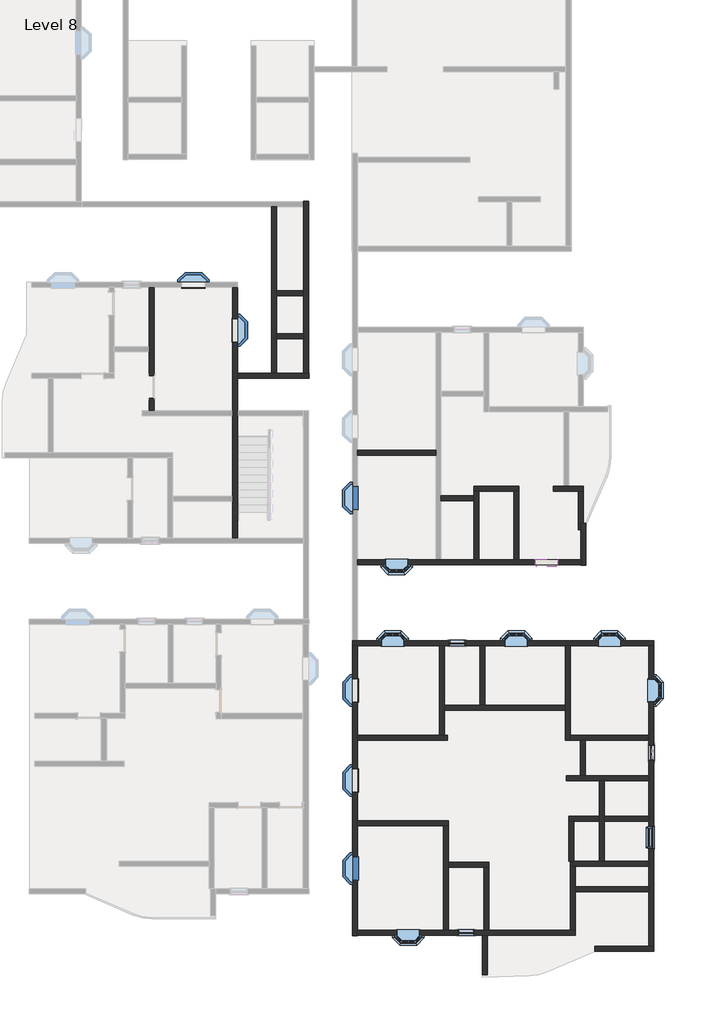
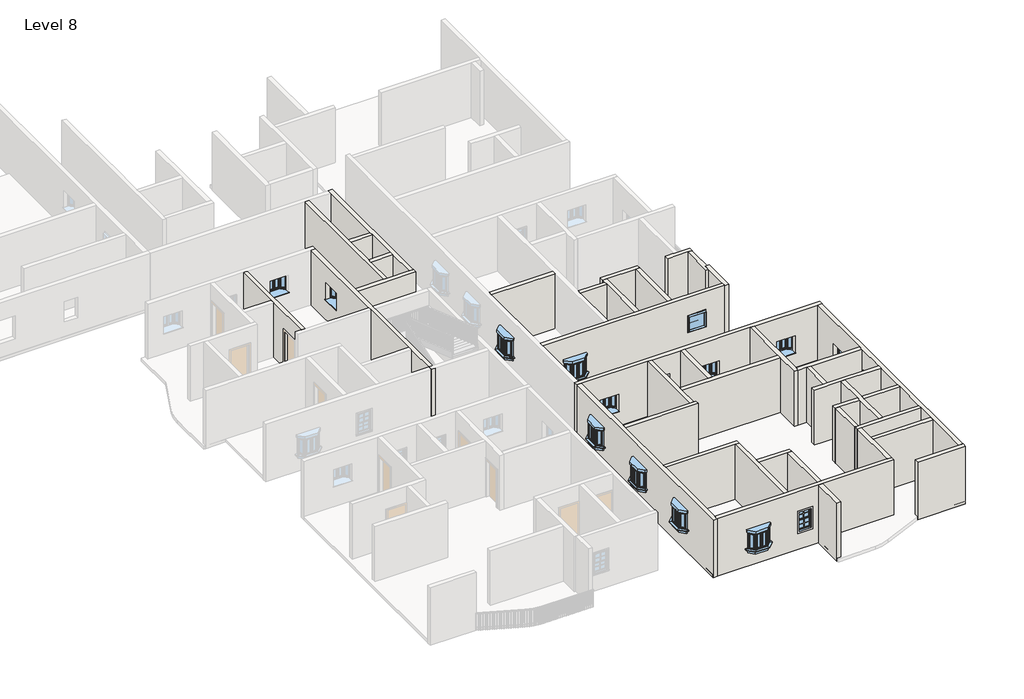
# One storey, part 2 of 14: 40 walls, 17 windows.
# Revit data of these elements (continued)
# Element 43 (IfcWindow, "910x910mm")
#   Mark = "444"
#   Phase Created = New Construction
#   Materials on its faces: "Window Frame", "Glass"
# Element 44 (IfcWindow, "910x910mm")
#   Mark = "435"
#   Phase Created = New Construction
#   Materials on its faces: "Window Frame", "Glass"
# Element 45 (IfcWindow, "910x910mm")
#   Mark = "436"
#   Phase Created = New Construction
#   Materials on its faces: "Window Frame", "Glass"
# Element 46 (IfcWindow, "910x910mm")
#   Mark = "437"
#   Phase Created = New Construction
#   Materials on its faces: "Window Frame", "Glass"
# Element 47 (IfcWindow, "910x910mm")
#   Mark = "438"
#   Phase Created = New Construction
#   Materials on its faces: "Window Frame", "Glass"
# Element 48 (IfcWindow, "910x910mm")
#   Mark = "439"
#   Phase Created = New Construction
#   Materials on its faces: "Window Frame", "Glass"
# Element 49 (IfcWindow, "910x910mm")
#   Mark = "440"
#   Phase Created = New Construction
#   Materials on its faces: "Window Frame", "Glass"
# Element 50 (IfcWindow, "910x910mm")
#   Mark = "441"
#   Phase Created = New Construction
#   Materials on its faces: "Window Frame", "Glass"
# Element 51 (IfcWindow, "910x910mm")
#   Mark = "442"
#   Phase Created = New Construction
#   Materials on its faces: "Window Frame", "Glass"
# Element 52 (IfcWindow, "910x910mm")
#   Mark = "443"
#   Phase Created = New Construction
#   Materials on its faces: "Window Frame", "Glass"
# Element 53 (IfcWindow, "Window-Double-Hung : 26\" x 42\"")
#   Mark = "466"
#   Window Inset = 0' - 0"
#   Interior Wall Closure = 0' - 1 1/2"
#   Frame Extension = 0' - 1 1/4"
#   Exterior Wall Closure = 0' - 0 1/2"
#   Interior Trim Visibility = yes
#   Indicator Visibility = yes
#   Exterior Trim Visibility = yes
#   Phase Created = New Construction
#   Materials on its faces: "Wood - Stained", "Glass", "Clad - White"
# Element 54 (IfcWindow, "Window-Double-Hung : 26\" x 42\"")
#   Mark = "467"
#   Window Inset = 0' - 0"
#   Interior Wall Closure = 0' - 1 1/2"
#   Frame Extension = 0' - 1 1/4"
#   Exterior Wall Closure = 0' - 0 1/2"
#   Interior Trim Visibility = yes
#   Indicator Visibility = yes
#   Exterior Trim Visibility = yes
#   Phase Created = New Construction
#   Materials on its faces: "Wood - Stained", "Glass", "Clad - White"
# Element 55 (IfcWindow, "Window-Double-Hung : 26\" x 42\"")
#   Mark = "468"
#   Window Inset = 0' - 0"
#   Interior Wall Closure = 0' - 1 1/2"
#   Frame Extension = 0' - 1 1/4"
#   Exterior Wall Closure = 0' - 0 1/2"
#   Interior Trim Visibility = yes
#   Indicator Visibility = yes
#   Exterior Trim Visibility = yes
#   Phase Created = New Construction
#   Materials on its faces: "Wood - Stained", "Glass", "Clad - White"
# Element 56 (IfcWindow, "Windows_Sgl_w-Glazing_Bars : 910x910mm")
#   Mark = "456"
#   Phase Created = New Construction
#   Materials on its faces: "Window Frame", "Glass"
# Element 57 (IfcWindow, "Windows_Sgl_w-Glazing_Bars : 910x910mm")
#   Mark = "455"
#   Phase Created = New Construction
#   Materials on its faces: "Window Frame", "Glass"
# Materials
#   "Window Frame": colour RGB 249 249 249, transparency 0
#   "Glass": class "Glass", colour RGB 0 128 192, transparency 0.75, Description = "Soda Lime Glass", Cost = 0
#   "Wood - Stained": class "Wood", colour RGB 224 178 126, transparency 0, Cost = 0
#   "Clad - White": class "Wood", colour RGB 242 242 238, transparency 0, Cost = 0
#   "Default Wall": colour RGB 128 128 128, transparency 0, Cost = 0
#   "Door - Frame": colour RGB 118 70 51, transparency 0, Cost = 0
#   "Acoustic Ceiling Tile 24 x 24": class "Generic", colour RGB 232 232 232, transparency 0, Description = "Acoustic Ceiling Tile 24 x 24", Cost = 0
#   "Earth": class "Generic", colour RGB 97 75 62, transparency 0, Description = "Soil", Cost = 0
#   "Carpet (1)": class "Carpet", colour RGB 124 80 67, transparency 0, Description = "Interior finish", Cost = 0
